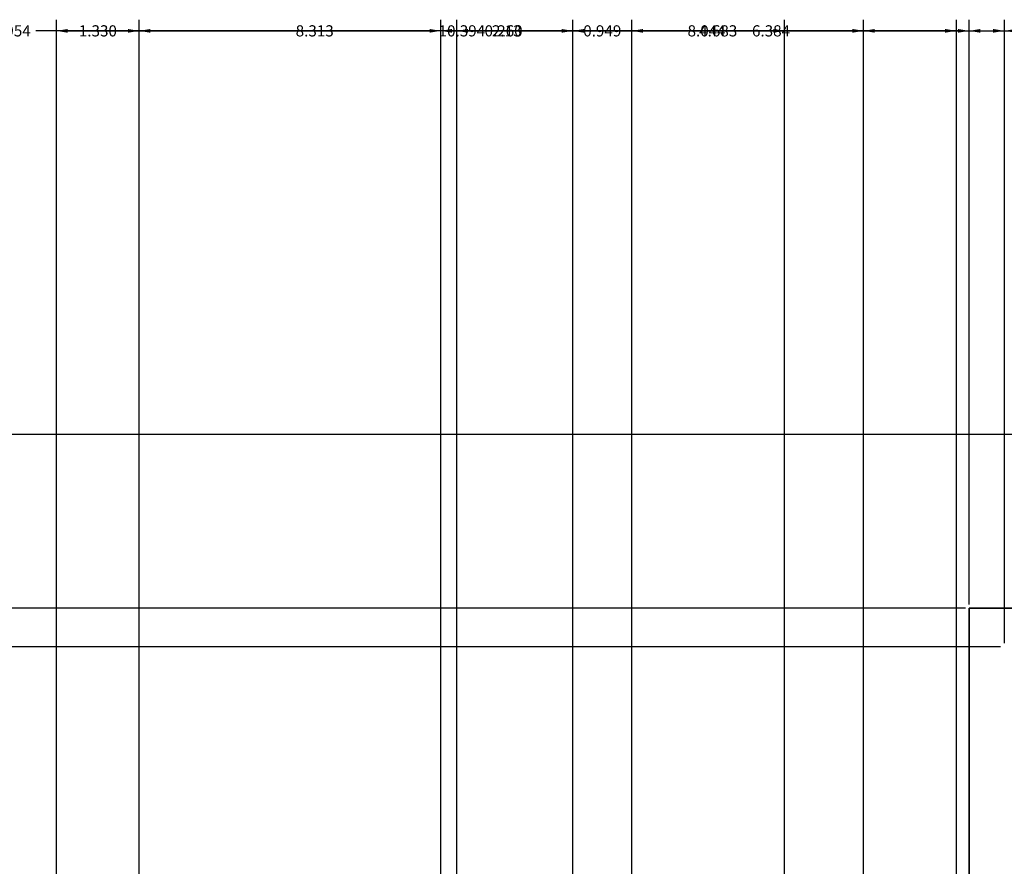
# Model space of a CAD drawing. Units: inches. Extents: x -10 to 130, y -32 to 34.
# Tile 8 of 22: x 12.81 to 28.66, y 20.25 to 33.88. Entities that reach past the tile are written whole.
import ezdxf

# ---------------------------------------------------------------- set-up
doc = ezdxf.new("R2010")
doc.units = ezdxf.units.IN
doc.header["$MEASUREMENT"] = 0
doc.layers.add('A-ANNO-DIMS', color=2, linetype='Continuous', lineweight=18)
doc.layers.add('A-ELEV', color=7, linetype='Continuous', lineweight=35)
doc.styles.get("Standard").update_dxf_attribs({"font": 'arial.ttf'})
doc.dimstyles.get("Standard").update_dxf_attribs({"dimtxt": 0.18, "dimasz": 0.18, "dimexe": 0.18, "dimexo": 0.0625, "dimgap": 0.09, "dimtad": 0, "dimtih": 1, "dimtoh": 1, "dimdec": 4, "dimzin": 0, "dimdsep": 46, "dimtxsty": 'Standard', "dimcen": 0.09, "dimadec": 0, "dimazin": 0, "dimtfac": 1, "dimtdec": 4, "dimtofl": 0, "dimtmove": 0, "dimatfit": 3, "dimfxl": 1, "dimtolj": 1, "dimtzin": 0, "dimarcsym": 0})

# ---------------------------------------------------------------- blocks, each defined once
blk = doc.blocks.new('*D3')
at = {"layer": 'A-ANNO-DIMS', "color": 0, "lineweight": -2, "transparency": 16777216}
for p, q in [((13.402, 6.07), (13.402, 33.879)), ((21.715, 6.07), (21.715, 33.879)), ((13.582, 33.699), (17.165, 33.699)), ((21.535, 33.699), (17.953, 33.699))]:
    blk.add_line(p, q, dxfattribs=at)
at = {"layer": 'A-ANNO-DIMS', "color": 0, "transparency": 16777216}
for points in [[(13.582, 33.729), (13.582, 33.669), (13.402, 33.699)], [(21.535, 33.729), (21.535, 33.669), (21.715, 33.699)]]:
    blk.add_solid(points, dxfattribs=at)
at = {"layer": 'Defpoints', "color": 0, "transparency": 16777216}
for p in [(21.715, 33.699), (13.402, 6.007), (21.715, 6.007)]:
    blk.add_point(p, dxfattribs=at)
at = {"layer": 'A-ANNO-DIMS', "color": 0, "transparency": 16777216, "insert": (17.559, 33.699), "char_height": 0.18, "attachment_point": 5}
blk.add_mtext('\\A1;8.313', dxfattribs=at)
blk = doc.blocks.new('*D4')
at = {"layer": 'A-ANNO-DIMS', "color": 0, "lineweight": -2, "transparency": 16777216}
for p, q in [((21.715, 6.07), (21.715, 33.879)), ((26.399, 6.07), (26.399, 33.879)), ((21.895, 33.699), (23.66, 33.699)), ((26.219, 33.699), (24.454, 33.699))]:
    blk.add_line(p, q, dxfattribs=at)
at = {"layer": 'A-ANNO-DIMS', "color": 0, "transparency": 16777216}
for points in [[(21.895, 33.729), (21.895, 33.669), (21.715, 33.699)], [(26.219, 33.729), (26.219, 33.669), (26.399, 33.699)]]:
    blk.add_solid(points, dxfattribs=at)
at = {"layer": 'Defpoints', "color": 0, "transparency": 16777216}
for p in [(26.399, 33.699), (21.715, 6.007), (26.399, 6.007)]:
    blk.add_point(p, dxfattribs=at)
at = {"layer": 'A-ANNO-DIMS', "color": 0, "transparency": 16777216, "insert": (24.057, 33.699), "char_height": 0.18, "attachment_point": 5}
blk.add_mtext('\\A1;4.683', dxfattribs=at)
blk = doc.blocks.new('*D5')
at = {"layer": 'A-ANNO-DIMS', "color": 0, "lineweight": -2, "transparency": 16777216}
for p, q in [((26.399, 6.07), (26.399, 33.879)), ((31.971, 6.07), (31.971, 33.879)), ((26.579, 33.699), (28.792, 33.699)), ((31.791, 33.699), (29.578, 33.699))]:
    blk.add_line(p, q, dxfattribs=at)
at = {"layer": 'A-ANNO-DIMS', "color": 0, "transparency": 16777216}
for points in [[(26.579, 33.729), (26.579, 33.669), (26.399, 33.699)], [(31.791, 33.729), (31.791, 33.669), (31.971, 33.699)]]:
    blk.add_solid(points, dxfattribs=at)
at = {"layer": 'Defpoints', "color": 0, "transparency": 16777216}
for p in [(31.971, 33.699), (26.399, 6.007), (31.971, 6.007)]:
    blk.add_point(p, dxfattribs=at)
at = {"layer": 'A-ANNO-DIMS', "color": 0, "transparency": 16777216, "insert": (29.185, 33.699), "char_height": 0.18, "attachment_point": 5}
blk.add_mtext('\\A1;5.572', dxfattribs=at)
blk = doc.blocks.new('*D11')
at = {"layer": 'A-ANNO-DIMS', "color": 0, "lineweight": -2, "transparency": 16777216}
for p, q in [((5.634, -12.739), (5.634, 33.879)), ((19.588, 19.547), (19.588, 33.879)), ((5.814, 33.699), (12.156, 33.699)), ((19.408, 33.699), (13.066, 33.699))]:
    blk.add_line(p, q, dxfattribs=at)
at = {"layer": 'A-ANNO-DIMS', "color": 0, "transparency": 16777216}
for points in [[(5.814, 33.729), (5.814, 33.669), (5.634, 33.699)], [(19.408, 33.729), (19.408, 33.669), (19.588, 33.699)]]:
    blk.add_solid(points, dxfattribs=at)
at = {"layer": 'Defpoints', "color": 0, "transparency": 16777216}
for p in [(19.588, 33.699), (19.588, 19.485), (5.634, -12.801)]:
    blk.add_point(p, dxfattribs=at)
at = {"layer": 'A-ANNO-DIMS', "color": 0, "transparency": 16777216, "insert": (12.611, 33.699), "char_height": 0.18, "attachment_point": 5}
blk.add_mtext('\\A1;13.954', dxfattribs=at)
blk = doc.blocks.new('*D12')
at = {"layer": 'A-ANNO-DIMS', "color": 0, "lineweight": -2, "transparency": 16777216}
for p, q in [((19.588, 19.547), (19.588, 33.879)), ((21.715, 14.903), (21.715, 33.879)), ((19.768, 33.699), (20.326, 33.699)), ((21.535, 33.699), (20.977, 33.699))]:
    blk.add_line(p, q, dxfattribs=at)
at = {"layer": 'A-ANNO-DIMS', "color": 0, "transparency": 16777216}
for points in [[(19.768, 33.729), (19.768, 33.669), (19.588, 33.699)], [(21.535, 33.729), (21.535, 33.669), (21.715, 33.699)]]:
    blk.add_solid(points, dxfattribs=at)
at = {"layer": 'Defpoints', "color": 0, "transparency": 16777216}
for p in [(21.715, 33.699), (19.588, 19.485), (21.715, 14.841)]:
    blk.add_point(p, dxfattribs=at)
at = {"layer": 'A-ANNO-DIMS', "color": 0, "transparency": 16777216, "insert": (20.652, 33.699), "char_height": 0.18, "attachment_point": 5}
blk.add_mtext('\\A1;2.13', dxfattribs=at)
blk = doc.blocks.new('*D13')
at = {"layer": 'A-ANNO-DIMS', "color": 0, "lineweight": -2, "transparency": 16777216}
for p, q in [((21.715, 14.903), (21.715, 33.879)), ((28.1, 24.464), (28.1, 33.879)), ((21.895, 33.699), (24.514, 33.699)), ((27.92, 33.699), (25.301, 33.699))]:
    blk.add_line(p, q, dxfattribs=at)
at = {"layer": 'A-ANNO-DIMS', "color": 0, "transparency": 16777216}
for points in [[(21.895, 33.729), (21.895, 33.669), (21.715, 33.699)], [(27.92, 33.729), (27.92, 33.669), (28.1, 33.699)]]:
    blk.add_solid(points, dxfattribs=at)
at = {"layer": 'Defpoints', "color": 0, "transparency": 16777216}
for p in [(28.1, 33.699), (28.1, 24.402), (21.715, 14.841)]:
    blk.add_point(p, dxfattribs=at)
at = {"layer": 'A-ANNO-DIMS', "color": 0, "transparency": 16777216, "insert": (24.908, 33.699), "char_height": 0.18, "attachment_point": 5}
blk.add_mtext('\\A1;6.384', dxfattribs=at)
blk = doc.blocks.new('*D14')
at = {"layer": 'A-ANNO-DIMS', "color": 0, "lineweight": -2, "transparency": 16777216}
for p, q in [((28.1, 24.464), (28.1, 33.879)), ((33.608, 19.52), (33.608, 33.879)), ((28.28, 33.699), (30.46, 33.699)), ((33.428, 33.699), (31.248, 33.699))]:
    blk.add_line(p, q, dxfattribs=at)
at = {"layer": 'A-ANNO-DIMS', "color": 0, "transparency": 16777216}
for points in [[(28.28, 33.729), (28.28, 33.669), (28.1, 33.699)], [(33.428, 33.729), (33.428, 33.669), (33.608, 33.699)]]:
    blk.add_solid(points, dxfattribs=at)
at = {"layer": 'Defpoints', "color": 0, "transparency": 16777216}
for p in [(33.608, 33.699), (28.1, 24.402), (33.608, 19.458)]:
    blk.add_point(p, dxfattribs=at)
at = {"layer": 'A-ANNO-DIMS', "color": 0, "transparency": 16777216, "insert": (30.854, 33.699), "char_height": 0.18, "attachment_point": 5}
blk.add_mtext('\\A1;5.508', dxfattribs=at)
blk = doc.blocks.new('*D28')
at = {"layer": 'A-ANNO-DIMS', "color": 0, "lineweight": -2, "transparency": 16777216}
for p, q in [((21.715, 14.903), (21.715, 33.879)), ((49.946, 14.903), (49.946, 33.879)), ((21.895, 33.699), (35.436, 33.699)), ((49.766, 33.699), (36.226, 33.699))]:
    blk.add_line(p, q, dxfattribs=at)
at = {"layer": 'A-ANNO-DIMS', "color": 0, "transparency": 16777216}
for points in [[(21.895, 33.729), (21.895, 33.669), (21.715, 33.699)], [(49.766, 33.729), (49.766, 33.669), (49.946, 33.699)]]:
    blk.add_solid(points, dxfattribs=at)
at = {"layer": 'Defpoints', "color": 0, "transparency": 16777216}
for p in [(49.946, 33.699), (21.715, 14.841), (49.946, 14.841)]:
    blk.add_point(p, dxfattribs=at)
at = {"layer": 'A-ANNO-DIMS', "color": 0, "transparency": 16777216, "insert": (35.831, 33.699), "char_height": 0.18, "attachment_point": 5}
blk.add_mtext('\\A1;28.23', dxfattribs=at)
blk = doc.blocks.new('*D38')
at = {"layer": 'A-ANNO-DIMS', "color": 0, "lineweight": -2, "transparency": 16777216}
for p, q in [((28.037, 24.402), (-9.564, 24.402)), ((-9.384, 24.222), (-9.384, 22.125)), ((-9.384, 19.665), (-9.384, 21.761)), ((19.526, 19.485), (-9.564, 19.485))]:
    blk.add_line(p, q, dxfattribs=at)
at = {"layer": 'A-ANNO-DIMS', "color": 0, "transparency": 16777216}
for points in [[(-9.414, 24.222), (-9.354, 24.222), (-9.384, 24.402)], [(-9.414, 19.665), (-9.354, 19.665), (-9.384, 19.485)]]:
    blk.add_solid(points, dxfattribs=at)
at = {"layer": 'Defpoints', "color": 0, "transparency": 16777216}
for p in [(-9.384, 24.402), (28.1, 24.402), (19.588, 19.485)]:
    blk.add_point(p, dxfattribs=at)
at = {"layer": 'A-ANNO-DIMS', "color": 0, "transparency": 16777216, "insert": (-9.384, 21.943), "char_height": 0.18, "attachment_point": 5}
blk.add_mtext('\\A1;4.917', dxfattribs=at)
blk = doc.blocks.new('*D39')
at = {"layer": 'A-ANNO-DIMS', "color": 0, "lineweight": -2, "transparency": 16777216}
for p, q in [((49.972, 27.199), (-9.564, 27.199)), ((-9.384, 27.019), (-9.384, 25.982)), ((-9.384, 24.582), (-9.384, 25.618)), ((28.037, 24.402), (-9.564, 24.402))]:
    blk.add_line(p, q, dxfattribs=at)
at = {"layer": 'A-ANNO-DIMS', "color": 0, "transparency": 16777216}
for points in [[(-9.414, 27.019), (-9.354, 27.019), (-9.384, 27.199)], [(-9.414, 24.582), (-9.354, 24.582), (-9.384, 24.402)]]:
    blk.add_solid(points, dxfattribs=at)
at = {"layer": 'Defpoints', "color": 0, "transparency": 16777216}
for p in [(-9.384, 27.199), (50.035, 27.199), (28.1, 24.402)]:
    blk.add_point(p, dxfattribs=at)
at = {"layer": 'A-ANNO-DIMS', "color": 0, "transparency": 16777216, "insert": (-9.384, 25.8), "char_height": 0.18, "attachment_point": 5}
blk.add_mtext('\\A1;2.797', dxfattribs=at)
blk = doc.blocks.new('*D96')
at = {"layer": 'A-ANNO-DIMS', "color": 0, "lineweight": -2, "transparency": 16777216}
for p, q in [((19.588, 19.547), (19.588, 33.879)), ((19.848, 19.232), (19.848, 33.879)), ((19.408, 33.699), (19.228, 33.699)), ((20.028, 33.699), (20.208, 33.699))]:
    blk.add_line(p, q, dxfattribs=at)
at = {"layer": 'A-ANNO-DIMS', "color": 0, "transparency": 16777216}
for points in [[(19.408, 33.729), (19.408, 33.669), (19.588, 33.699)], [(20.028, 33.729), (20.028, 33.669), (19.848, 33.699)]]:
    blk.add_solid(points, dxfattribs=at)
at = {"layer": 'Defpoints', "color": 0, "transparency": 16777216}
for p in [(19.848, 33.699), (19.588, 19.485), (19.848, 19.17)]:
    blk.add_point(p, dxfattribs=at)
at = {"layer": 'A-ANNO-DIMS', "color": 0, "transparency": 16777216, "insert": (20.601, 33.699), "char_height": 0.18, "attachment_point": 5}
blk.add_mtext('\\A1;0.260', dxfattribs=at)
blk = doc.blocks.new('*D97')
at = {"layer": 'A-ANNO-DIMS', "color": 0, "lineweight": -2, "transparency": 16777216}
for p, q in [((19.848, 19.232), (19.848, 33.879)), ((27.892, 19.232), (27.892, 33.879)), ((20.028, 33.699), (23.476, 33.699)), ((27.712, 33.699), (24.263, 33.699))]:
    blk.add_line(p, q, dxfattribs=at)
at = {"layer": 'A-ANNO-DIMS', "color": 0, "transparency": 16777216}
for points in [[(20.028, 33.729), (20.028, 33.669), (19.848, 33.699)], [(27.712, 33.729), (27.712, 33.669), (27.892, 33.699)]]:
    blk.add_solid(points, dxfattribs=at)
at = {"layer": 'Defpoints', "color": 0, "transparency": 16777216}
for p in [(27.892, 33.699), (19.848, 19.17), (27.892, 19.17)]:
    blk.add_point(p, dxfattribs=at)
at = {"layer": 'A-ANNO-DIMS', "color": 0, "transparency": 16777216, "insert": (23.87, 33.699), "char_height": 0.18, "attachment_point": 5}
blk.add_mtext('\\A1;8.044', dxfattribs=at)
blk = doc.blocks.new('*D99')
at = {"layer": 'A-ANNO-DIMS', "color": 0, "lineweight": -2, "transparency": 16777216}
for p, q in [((28.1, 24.464), (28.1, 33.879)), ((28.665, 23.841), (28.665, 33.879)), ((28.28, 33.699), (28.485, 33.699)), ((28.665, 33.699), (28.845, 33.699))]:
    blk.add_line(p, q, dxfattribs=at)
at = {"layer": 'A-ANNO-DIMS', "color": 0, "transparency": 16777216}
for points in [[(28.28, 33.729), (28.28, 33.669), (28.1, 33.699)], [(28.485, 33.729), (28.485, 33.669), (28.665, 33.699)]]:
    blk.add_solid(points, dxfattribs=at)
at = {"layer": 'Defpoints', "color": 0, "transparency": 16777216}
for p in [(28.665, 33.699), (28.1, 24.402), (28.665, 23.779)]:
    blk.add_point(p, dxfattribs=at)
at = {"layer": 'A-ANNO-DIMS', "color": 0, "transparency": 16777216, "insert": (29.239, 33.699), "char_height": 0.18, "attachment_point": 5}
blk.add_mtext('\\A1;0.565', dxfattribs=at)
blk = doc.blocks.new('*D100')
at = {"layer": 'A-ANNO-DIMS', "color": 0, "lineweight": -2, "transparency": 16777216}
for p, q in [((28.665, 23.841), (28.665, 33.879)), ((35.841, 23.841), (35.841, 33.879)), ((28.845, 33.699), (31.86, 33.699)), ((35.661, 33.699), (32.646, 33.699))]:
    blk.add_line(p, q, dxfattribs=at)
at = {"layer": 'A-ANNO-DIMS', "color": 0, "transparency": 16777216}
for points in [[(28.845, 33.729), (28.845, 33.669), (28.665, 33.699)], [(35.661, 33.729), (35.661, 33.669), (35.841, 33.699)]]:
    blk.add_solid(points, dxfattribs=at)
at = {"layer": 'Defpoints', "color": 0, "transparency": 16777216}
for p in [(35.841, 33.699), (28.665, 23.779), (35.841, 23.779)]:
    blk.add_point(p, dxfattribs=at)
at = {"layer": 'A-ANNO-DIMS', "color": 0, "transparency": 16777216, "insert": (32.253, 33.699), "char_height": 0.18, "attachment_point": 5}
blk.add_mtext('\\A1;7.176', dxfattribs=at)
blk = doc.blocks.new('*D101')
at = {"layer": 'A-ANNO-DIMS', "color": 0, "lineweight": -2, "transparency": 16777216}
for p, q in [((-9.384, 24.402), (-9.384, 24.582)), ((-9.384, 24.582), (-9.204, 24.582)), ((28.037, 24.402), (-9.564, 24.402)), ((-9.384, 23.959), (-9.384, 24.222)), ((28.602, 23.779), (-9.564, 23.779))]:
    blk.add_line(p, q, dxfattribs=at)
at = {"layer": 'A-ANNO-DIMS', "color": 0, "transparency": 16777216}
for points in [[(-9.414, 24.222), (-9.354, 24.222), (-9.384, 24.402)], [(-9.414, 23.959), (-9.354, 23.959), (-9.384, 23.779)]]:
    blk.add_solid(points, dxfattribs=at)
at = {"layer": 'Defpoints', "color": 0, "transparency": 16777216}
for p in [(-9.384, 24.402), (28.1, 24.402), (28.665, 23.779)]:
    blk.add_point(p, dxfattribs=at)
at = {"layer": 'A-ANNO-DIMS', "color": 0, "transparency": 16777216, "insert": (-8.81, 24.582), "char_height": 0.18, "attachment_point": 5}
blk.add_mtext('\\A1;0.623', dxfattribs=at)
blk = doc.blocks.new('*D105')
at = {"layer": 'A-ANNO-DIMS', "color": 0, "lineweight": -2, "transparency": 16777216}
for p, q in [((21.715452, 14.90344), (21.715452, 33.878656)), ((22.664856, 14.318095), (22.664856, 33.878656)), ((21.535452, 33.698656), (21.355452, 33.698656)), ((22.844856, 33.698656), (23.024856, 33.698656))]:
    blk.add_line(p, q, dxfattribs=at)
at = {"layer": 'A-ANNO-DIMS', "color": 0, "transparency": 16777216}
for points in [[(21.535452, 33.728656), (21.535452, 33.668656), (21.715452, 33.698656)], [(22.844856, 33.728656), (22.844856, 33.668656), (22.664856, 33.698656)]]:
    blk.add_solid(points, dxfattribs=at)
at = {"layer": 'Defpoints', "color": 0, "transparency": 16777216}
for p in [(22.664856, 33.698656), (21.715452, 14.84094), (22.664856, 14.255595)]:
    blk.add_point(p, dxfattribs=at)
at = {"layer": 'A-ANNO-DIMS', "color": 0, "transparency": 16777216, "insert": (22.190154, 33.698656), "char_height": 0.18, "attachment_point": 5}
blk.add_mtext('\\A1;0.949', dxfattribs=at)
blk = doc.blocks.new('*D106')
at = {"layer": 'A-ANNO-DIMS', "color": 0, "lineweight": -2, "transparency": 16777216}
for p, q in [((22.665, 14.318), (22.665, 33.879)), ((48.963, 14.318), (48.963, 33.879)), ((22.845, 33.699), (35.349, 33.699)), ((48.783, 33.699), (36.279, 33.699))]:
    blk.add_line(p, q, dxfattribs=at)
at = {"layer": 'A-ANNO-DIMS', "color": 0, "transparency": 16777216}
for points in [[(22.845, 33.729), (22.845, 33.669), (22.665, 33.699)], [(48.783, 33.729), (48.783, 33.669), (48.963, 33.699)]]:
    blk.add_solid(points, dxfattribs=at)
at = {"layer": 'Defpoints', "color": 0, "transparency": 16777216}
for p in [(48.963, 33.699), (22.665, 14.256), (48.963, 14.256)]:
    blk.add_point(p, dxfattribs=at)
at = {"layer": 'A-ANNO-DIMS', "color": 0, "transparency": 16777216, "insert": (35.814, 33.699), "char_height": 0.18, "attachment_point": 5}
blk.add_mtext('\\A1;26.298', dxfattribs=at)
blk = doc.blocks.new('*D111')
at = {"layer": 'A-ANNO-DIMS', "color": 0, "lineweight": -2, "transparency": 16777216}
for p, q in [((13.402, 6.07), (13.402, 33.879)), ((14.732, 5.012), (14.732, 33.879)), ((13.582, 33.699), (13.682, 33.699)), ((14.552, 33.699), (14.452, 33.699))]:
    blk.add_line(p, q, dxfattribs=at)
at = {"layer": 'A-ANNO-DIMS', "color": 0, "transparency": 16777216}
for points in [[(13.582, 33.729), (13.582, 33.669), (13.402, 33.699)], [(14.552, 33.729), (14.552, 33.669), (14.732, 33.699)]]:
    blk.add_solid(points, dxfattribs=at)
at = {"layer": 'Defpoints', "color": 0, "transparency": 16777216}
for p in [(14.732, 33.699), (13.402, 6.007), (14.732, 4.95)]:
    blk.add_point(p, dxfattribs=at)
at = {"layer": 'A-ANNO-DIMS', "color": 0, "transparency": 16777216, "insert": (14.067, 33.699), "char_height": 0.18, "attachment_point": 5}
blk.add_mtext('\\A1;1.330', dxfattribs=at)
blk = doc.blocks.new('*D112')
at = {"layer": 'A-ANNO-DIMS', "color": 0, "lineweight": -2, "transparency": 16777216}
for p, q in [((14.732, 5.012), (14.732, 33.879)), ((25.126, 5.012), (25.126, 33.879)), ((14.912, 33.699), (19.474, 33.699)), ((24.946, 33.699), (20.384, 33.699))]:
    blk.add_line(p, q, dxfattribs=at)
at = {"layer": 'A-ANNO-DIMS', "color": 0, "transparency": 16777216}
for points in [[(14.912, 33.729), (14.912, 33.669), (14.732, 33.699)], [(24.946, 33.729), (24.946, 33.669), (25.126, 33.699)]]:
    blk.add_solid(points, dxfattribs=at)
at = {"layer": 'Defpoints', "color": 0, "transparency": 16777216}
for p in [(25.126, 33.699), (14.732, 4.95), (25.126, 4.95)]:
    blk.add_point(p, dxfattribs=at)
at = {"layer": 'A-ANNO-DIMS', "color": 0, "transparency": 16777216, "insert": (19.929, 33.699), "char_height": 0.18, "attachment_point": 5}
blk.add_mtext('\\A1;10.394', dxfattribs=at)

msp = doc.modelspace()

# ---------------------------------------------------------------- linework, layer by layer
at = {"layer": 'A-ELEV'}
for p, q in [((28.0997, 18.6807), (28.0997, 24.4019)), ((28.0997, 24.4019), (36.3774, 24.4019))]:
    msp.add_line(p, q, dxfattribs=at)

# ---------------------------------------------------------------- dimensions: what is measured, and where the dimension line sits
at = {"layer": 'A-ANNO-DIMS'}
for base, p1, p2, override, picture, middle in [((19.5881, 33.6987), (5.634, -12.8012), (19.5881, 19.4845), {"dimdec": 3, "dimlfac": 1, "dimrnd": 0, "dimzin": 0, "dimdsep": 46, "dimlunit": 2}, '*D11', (12.611, 33.6987)), ((21.7155, 33.6987), (13.4021, 6.0074), (21.7155, 6.0074), {"dimdec": 3, "dimlfac": 1, "dimrnd": 0, "dimzin": 0, "dimdsep": 46, "dimlunit": 2}, '*D3', (17.5588, 33.6987)), ((14.7324, 33.6987), (13.4021, 6.0074), (14.7324, 4.9495), {"dimdec": 3, "dimlfac": 1, "dimrnd": 0, "dimzin": 0, "dimdsep": 46, "dimlunit": 2}, '*D111', (14.0673, 33.6987)), ((25.1261, 33.6987), (14.7324, 4.9495), (25.1261, 4.9495), {"dimdec": 3, "dimlfac": 1, "dimrnd": 0, "dimzin": 0, "dimdsep": 46, "dimlunit": 2}, '*D112', (19.9293, 33.6987)), ((19.8477, 33.6987), (19.5881, 19.4845), (19.8477, 19.1697), {"dimdec": 3, "dimlfac": 1, "dimrnd": 0, "dimzin": 0, "dimdsep": 46, "dimlunit": 2}, '*D96', (20.6011, 33.6987)), ((21.7155, 33.6987), (19.5881, 19.4845), (21.7155, 14.8409), {"dimdec": 2, "dimlfac": 1, "dimrnd": 0, "dimzin": 0, "dimdsep": 46, "dimlunit": 2}, '*D12', (20.6518, 33.6987)), ((27.8916, 33.6987), (19.8477, 19.1697), (27.8916, 19.1697), {"dimdec": 3, "dimlfac": 1, "dimrnd": 0, "dimzin": 0, "dimdsep": 46, "dimlunit": 2}, '*D97', (23.8696, 33.6987)), ((22.6649, 33.6987), (21.7155, 14.8409), (22.6649, 14.2556), {"dimdec": 3, "dimlfac": 1, "dimrnd": 0, "dimzin": 0, "dimdsep": 46, "dimlunit": 2}, '*D105', (22.1902, 33.6987)), ((26.3988, 33.6987), (21.7155, 6.0074), (26.3988, 6.0074), {"dimdec": 3, "dimlfac": 1, "dimrnd": 0, "dimzin": 0, "dimdsep": 46, "dimlunit": 2}, '*D4', (24.0571, 33.6987)), ((28.0997, 33.6987), (21.7155, 14.8409), (28.0997, 24.4019), {"dimdec": 3, "dimlfac": 1, "dimrnd": 0, "dimzin": 0, "dimdsep": 46, "dimlunit": 2}, '*D13', (24.9076, 33.6987)), ((49.9462, 33.6987), (21.7155, 14.8409), (49.9462, 14.8409), {"dimdec": 2, "dimlfac": 1, "dimrnd": 0, "dimzin": 0, "dimdsep": 46, "dimlunit": 2}, '*D28', (35.8308, 33.6987)), ((48.963, 33.6987), (22.6649, 14.2556), (48.963, 14.2556), {"dimdec": 3, "dimlfac": 1, "dimrnd": 0, "dimzin": 0, "dimdsep": 46, "dimlunit": 2}, '*D106', (35.8139, 33.6987)), ((31.9712, 33.6987), (26.3988, 6.0074), (31.9712, 6.0074), {"dimdec": 3, "dimlfac": 1, "dimrnd": 0, "dimzin": 0, "dimdsep": 46, "dimlunit": 2}, '*D5', (29.185, 33.6987)), ((33.60816, 33.69866), (28.0997, 24.40191), (33.60816, 19.45752), {"dimdec": 3, "dimlfac": 1, "dimrnd": 0, "dimzin": 0, "dimdsep": 46, "dimlunit": 2}, '*D14', (30.85393, 33.69866)), ((28.6645, 33.6987), (28.0997, 24.4019), (28.6645, 23.7785), {"dimdec": 3, "dimlfac": 1, "dimrnd": 0, "dimzin": 0, "dimdsep": 46, "dimlunit": 2}, '*D99', (29.2389, 33.6987)), ((35.84098, 33.69866), (28.66453, 23.77854), (35.84098, 23.77854), {"dimdec": 3, "dimlfac": 1, "dimrnd": 0, "dimzin": 0, "dimdsep": 46, "dimlunit": 2}, '*D100', (32.25276, 33.69866))]:
    dim = msp.add_linear_dim(base=base, p1=p1, p2=p2, dimstyle='Standard', override=override, dxfattribs=at)
    dim.commit()
    dim.dimension.update_dxf_attribs({"geometry": picture, "text_midpoint": middle})
for base, p1, p2, picture, middle in [((-9.3836, 27.1987), (28.0997, 24.4019), (50.0347, 27.1987), '*D39', (-9.3836, 25.8003)), ((-9.3836, 24.4019), (28.6645, 23.7785), (28.0997, 24.4019), '*D101', (-8.8098, 24.5819)), ((-9.3836, 24.4019), (19.5881, 19.4845), (28.0997, 24.4019), '*D38', (-9.3836, 21.9432))]:
    dim = msp.add_linear_dim(base=base, p1=p1, p2=p2, angle=90, dimstyle='Standard', override={"dimdec": 3, "dimlfac": 1, "dimrnd": 0, "dimzin": 0, "dimdsep": 46, "dimlunit": 2}, dxfattribs=at)
    dim.commit()
    dim.dimension.update_dxf_attribs({"geometry": picture, "text_midpoint": middle})

doc.saveas('drawing.dxf')
